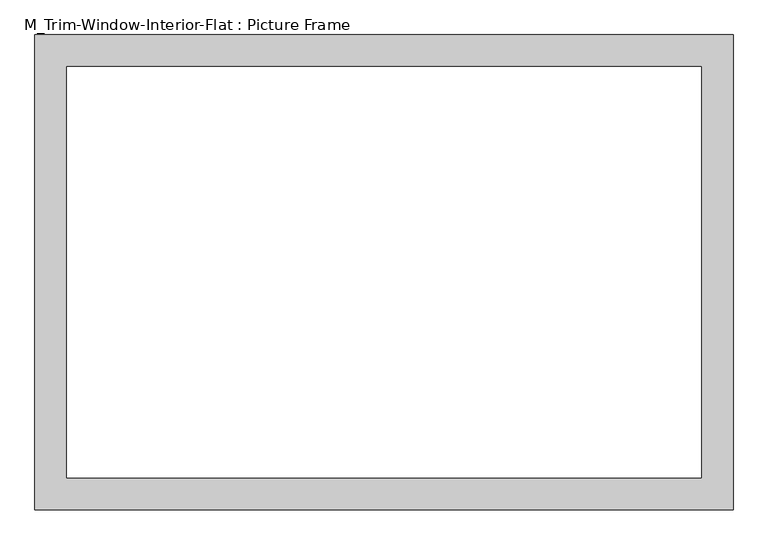
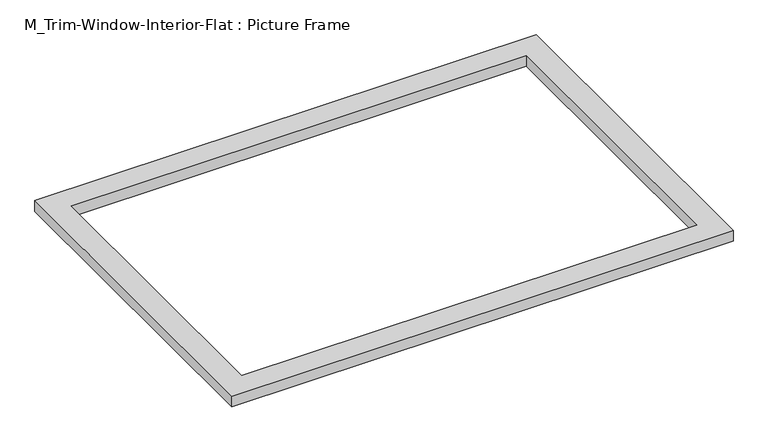
"""IFC4 building model written with IfcOpenShell, lengths in millimetres: proxy geometry, M_Trim-Window-Interior-Flat : Picture Frame."""

from ifc_helpers import new_model, si_unit, origin, origin_with_axes, place, context, project, spatial, polyline, outline, extrude, source, transform, mapped, element, save


def m_trim_window_interior_flat_picture_frame_580345df(model_context):
    return source(origin(), model_context, "Body", "SweptSolid", [
        extrude(outline(polyline([(656.9, 47.3), (656.9, -847.3), (-656.9, -847.3), (-656.9, 47.3), (656.9, 47.3)]), holes=[polyline([(596.9, -12.7), (-596.9, -12.7), (-596.9, -787.3), (596.9, -787.3), (596.9, -12.7)])]), origin_with_axes(), (0.0, 0.0, 1.0), 30.0),
    ])


if __name__ == "__main__":
    model = new_model("IFC4")
    model_context = context("Model", 3, world=origin())
    ifc_project = project(units=[si_unit("LENGTHUNIT", "METRE", prefix="MILLI")], contexts=[model_context])
    site = spatial("IfcSite", under=ifc_project)
    building = spatial("IfcBuilding", under=site)
    placement = place(None, origin())
    m_trim_window_interior_flat_picture_frame_shape = m_trim_window_interior_flat_picture_frame_580345df(model_context)
    element("IfcBuildingElementProxy", 1, Name="M_Trim-Window-Interior-Flat : Picture Frame", ObjectType="M_Trim-Window-Interior-Flat : Picture Frame", at=placement, inside=building, context=model_context, shape_type="MappedRepresentation", body=[
        mapped(m_trim_window_interior_flat_picture_frame_shape, transform((0.0, 0.0, 0.0), x_axis=(1.0, 0.0, 0.0), y_axis=(0.0, 1.0, 0.0), z_axis=(0.0, 0.0, 1.0))),
    ])
    save(model, "model.ifc")

# Revit data of these elements
# Type "M_Trim-Window-Interior-Flat : Picture Frame"
#   Trim Thickness_Picture Frame = 0' - 1.1811"
#   Trim Width = 0' - 2.3622"
#   Trim Thickness_with Sill = 0' - 0.7874"
#   Sill Thickness = 0' - 1.1811"
#   Opening Width [instance default] = 1' - 11.62205"
#   Opening Height [instance default] = 2' - 11.43307"
#   Default Elevation = 3' - 11.24409"
#   Sill = no
#   Picture Frame = yes
#   Trim Material [instance default] = none
# Element 1 (IfcBuildingElementProxy, "M_Trim-Window-Interior-Flat : Picture Frame")
#   Opening Width = 4' - 0"
#   Opening Height = 2' - 7.49606"
#   Trim Material = Wood - Stained
#   Materials on its faces: "Wood - Stained"
# Materials
#   "Wood - Stained": class "Wood", colour RGB 224 178 126, transparency 0, Cost = 0
